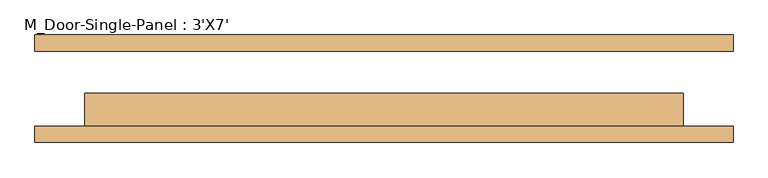
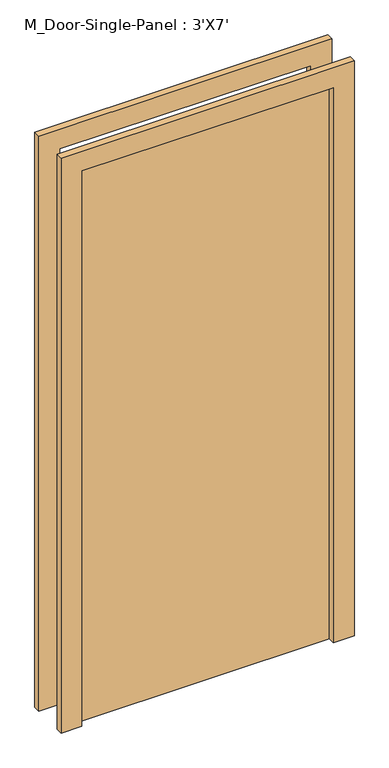
"""IFC4 building model written with IfcOpenShell, lengths in millimetres: door geometry, M_Door-Single-Panel : 3'X7'."""

from ifc_helpers import new_model, si_unit, frame, origin, origin_with_axes, place, context, project, spatial, polyline, outline, extrude, source, transform, mapped, element, save


def m_door_single_panel_3_x7_ebb67e73(model_context):
    return source(origin(), model_context, "Body", "SweptSolid", [
        extrude(outline(polyline([(457.2, -7.15), (457.2, -57.15), (-457.2, -57.15), (-457.2, -7.15), (457.2, -7.15)])), origin_with_axes(), (0.0, 0.0, 1.0), 2133.6),
        extrude(outline(polyline([(2209.8, 533.4), (2209.8, -533.4), (0.0, -533.4), (0.0, -457.2), (2133.6, -457.2), (2133.6, 457.2), (0.0, 457.2), (0.0, 533.4), (2209.8, 533.4)])), frame((0.0, 57.15, 0.0), z_axis=(0.0, 1.0, 0.0), x_axis=(0.0, 0.0, 1.0)), (0.0, 0.0, 1.0), 25.0),
        extrude(outline(polyline([(2209.8, -533.4), (0.0, -533.4), (0.0, -457.2), (2133.6, -457.2), (2133.6, 457.2), (0.0, 457.2), (0.0, 533.4), (2209.8, 533.4), (2209.8, -533.4)])), frame((0.0, -82.15, 0.0), z_axis=(0.0, 1.0, 0.0), x_axis=(0.0, 0.0, 1.0)), (0.0, 0.0, 1.0), 25.0),
    ])


if __name__ == "__main__":
    model = new_model("IFC4")
    model_context = context("Model", 3, world=origin())
    ifc_project = project(units=[si_unit("LENGTHUNIT", "METRE", prefix="MILLI")], contexts=[model_context])
    site = spatial("IfcSite", under=ifc_project)
    building = spatial("IfcBuilding", under=site)
    placement = place(None, origin())
    m_door_single_panel_3_x7_shape = m_door_single_panel_3_x7_ebb67e73(model_context)
    element("IfcDoor", 1, ObjectType="M_Door-Single-Panel : 3'X7'", at=placement, inside=building, context=model_context, shape_type="MappedRepresentation", body=[
        mapped(m_door_single_panel_3_x7_shape, transform((0.0, 0.0, 0.0), x_axis=(1.0, 0.0, 0.0), y_axis=(0.0, 1.0, 0.0), z_axis=(0.0, 0.0, 1.0))),
    ])
    save(model, "model.ifc")

# Revit data of these elements
# Type "M_Door-Single-Panel : 3'X7'"
#   Type Mark = "11"
#   Construction Type Id = "DOOR"
#   Assembly Code = "C1020300"
#   Analytic Construction = "Wooden"
#   Thickness = 0' - 1.9685"
#   Thermal Resistance (R) = 2.5876 (h·ft²·°F)/BTU
#   Swing Angle [instance default] = 90.00°
#   Heat Transfer Coefficient (U) = 0.3865 BTU/(h·ft²·°F)
#   Height = 7' - 0"
#   Trim Projection Ext = 0' - 0.98425"
#   Trim Projection Int = 0' - 0.98425"
#   Trim Width = 0' - 3.14961"
#   Width = 3' - 0"
#   Define Thermal Properties by = 1
#   Panel Material = Wood - Birch - Solid Stained Light Low Gloss
#   Trim Material = Paint - Sienna
#   Visual Light Transmittance = 0
#   Solar Heat Gain Coefficient = 0
#   Function = (empty or 0)
#   Wall Closure = (empty or 0)
# Element 1 (IfcDoor, "M_Door-Single-Panel : 3'X7'")
#   Materials on its faces: "Paint - Sienna", "Wood - Birch - Solid Stained Light Low Gloss"
# Materials
#   "Wood - Birch - Solid Stained Light Low Gloss": class "Wood", colour RGB 210 159 95, transparency 0, Cost = 0
#   "Paint - Sienna": colour RGB 118 70 51, transparency 0, Cost = 0
